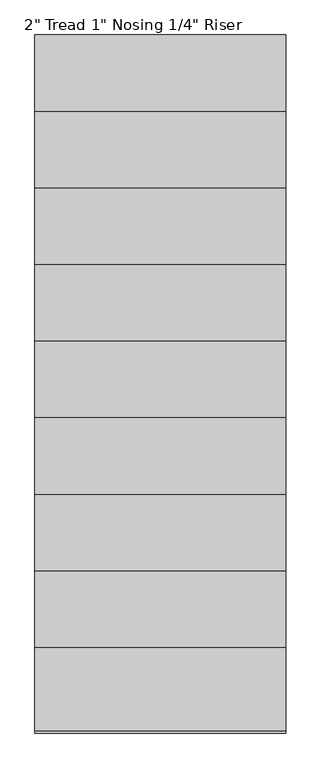
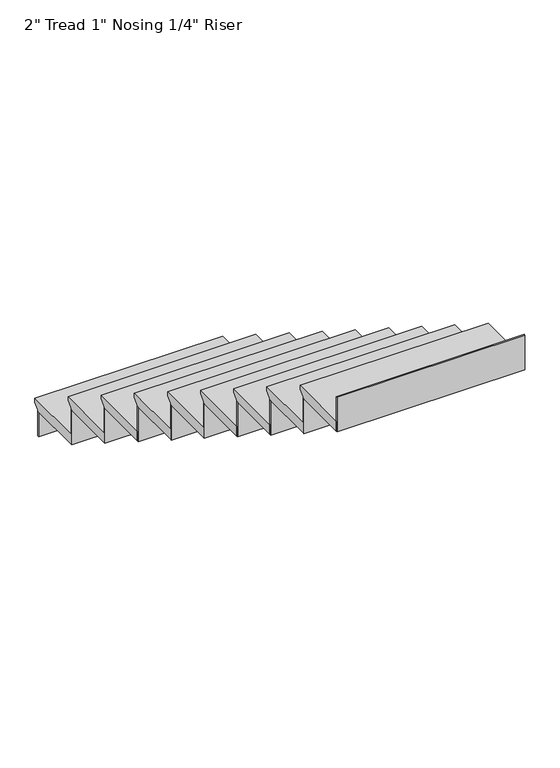
"""IFC4 building model written with IfcOpenShell, lengths in millimetres: stair flight geometry."""

from ifc_helpers import new_model, si_unit, origin, place, context, project, spatial, faceted_brep, source, transform, mapped, element, save


def stair_flight_2edfd720(model_context):
    return source(origin(), model_context, "Body", "Brep", [
        faceted_brep([(14235.8761273, -1100.1064015, 768.35), (14235.8761273, -1100.1064015, 787.4), (15150.2761273, -1100.1064015, 787.4), (15150.2761273, -1100.1064015, 768.35), (14235.8761273, -1125.5064015, 742.95), (15150.2761273, -1125.5064015, 742.95), (14235.8761273, -1404.9064015, 787.4), (15150.2761273, -1404.9064015, 787.4), (15150.2761273, -1125.5064015, 736.6), (15150.2761273, -1404.9064015, 736.6), (14235.8761273, -1404.9064015, 736.6), (14235.8761273, -1125.5064015, 736.6)], [[[0, 1, 2, 3]], [[4, 0, 3, 5]], [[2, 1, 6, 7]], [[8, 9, 10, 11]], [[2, 7, 9, 8, 5, 3]], [[8, 11, 4, 5]], [[6, 1, 0, 4, 11, 10]], [[7, 6, 10, 9]]]),
        faceted_brep([(14235.8761273, -1125.5064015, 736.6), (14235.8761273, -1125.5064015, 609.6), (14235.8761273, -1131.8564015, 609.6), (14235.8761273, -1131.8564015, 736.6), (15150.2761273, -1125.5064015, 736.6), (15150.2761273, -1131.8564015, 736.6), (15150.2761273, -1131.8564015, 609.6), (15150.2761273, -1125.5064015, 609.6)], [[[0, 1, 2, 3]], [[4, 5, 6, 7]], [[1, 0, 4, 7]], [[2, 1, 7, 6]], [[3, 2, 6, 5]], [[0, 3, 5, 4]]]),
        faceted_brep([(14235.8761273, -1404.9064015, 914.4), (14235.8761273, -1404.9064015, 736.6), (14235.8761273, -1411.2564015, 736.6), (14235.8761273, -1411.2564015, 914.4), (15150.2761273, -1404.9064015, 914.4), (15150.2761273, -1411.2564015, 914.4), (15150.2761273, -1411.2564015, 736.6), (15150.2761273, -1404.9064015, 736.6)], [[[0, 1, 2, 3]], [[4, 5, 6, 7]], [[1, 0, 4, 7]], [[2, 1, 7, 6]], [[3, 2, 6, 5]], [[0, 3, 5, 4]]]),
        faceted_brep([(15150.2761273, -1379.5064015, 965.2), (14235.8761273, -1379.5064015, 965.2), (14235.8761273, -1684.3064015, 965.2), (15150.2761273, -1684.3064015, 965.2), (15150.2761273, -1404.9064015, 914.4), (15150.2761273, -1684.3064015, 914.4), (14235.8761273, -1684.3064015, 914.4), (14235.8761273, -1404.9064015, 914.4), (15150.2761273, -1404.9064015, 920.75), (15150.2761273, -1379.5064015, 946.15), (14235.8761273, -1404.9064015, 920.75), (14235.8761273, -1379.5064015, 946.15)], [[[0, 1, 2, 3]], [[4, 5, 6, 7]], [[0, 3, 5, 4, 8, 9]], [[4, 7, 10, 8]], [[2, 1, 11, 10, 7, 6]], [[3, 2, 6, 5]], [[11, 1, 0, 9]], [[10, 11, 9, 8]]]),
        faceted_brep([(14235.8761273, -1684.3064015, 1092.2), (14235.8761273, -1684.3064015, 914.4), (14235.8761273, -1690.6564015, 914.4), (14235.8761273, -1690.6564015, 1092.2), (15150.2761273, -1684.3064015, 1092.2), (15150.2761273, -1690.6564015, 1092.2), (15150.2761273, -1690.6564015, 914.4), (15150.2761273, -1684.3064015, 914.4)], [[[0, 1, 2, 3]], [[4, 5, 6, 7]], [[1, 0, 4, 7]], [[2, 1, 7, 6]], [[3, 2, 6, 5]], [[0, 3, 5, 4]]]),
        faceted_brep([(15150.2761273, -1658.9064015, 1143.0), (14235.8761273, -1658.9064015, 1143.0), (14235.8761273, -1963.7064015, 1143.0), (15150.2761273, -1963.7064015, 1143.0), (15150.2761273, -1684.3064015, 1092.2), (15150.2761273, -1963.7064015, 1092.2), (14235.8761273, -1963.7064015, 1092.2), (14235.8761273, -1684.3064015, 1092.2), (15150.2761273, -1684.3064015, 1098.55), (15150.2761273, -1658.9064015, 1123.95), (14235.8761273, -1684.3064015, 1098.55), (14235.8761273, -1658.9064015, 1123.95)], [[[0, 1, 2, 3]], [[4, 5, 6, 7]], [[0, 3, 5, 4, 8, 9]], [[4, 7, 10, 8]], [[2, 1, 11, 10, 7, 6]], [[3, 2, 6, 5]], [[11, 1, 0, 9]], [[10, 11, 9, 8]]]),
        faceted_brep([(14235.8761273, -1963.7064015, 1270.0), (14235.8761273, -1963.7064015, 1092.2), (14235.8761273, -1970.0564015, 1092.2), (14235.8761273, -1970.0564015, 1270.0), (15150.2761273, -1963.7064015, 1270.0), (15150.2761273, -1970.0564015, 1270.0), (15150.2761273, -1970.0564015, 1092.2), (15150.2761273, -1963.7064015, 1092.2)], [[[0, 1, 2, 3]], [[4, 5, 6, 7]], [[1, 0, 4, 7]], [[2, 1, 7, 6]], [[3, 2, 6, 5]], [[0, 3, 5, 4]]]),
        faceted_brep([(15150.2761273, -1938.3064015, 1320.8), (14235.8761273, -1938.3064015, 1320.8), (14235.8761273, -2243.1064015, 1320.8), (15150.2761273, -2243.1064015, 1320.8), (15150.2761273, -1963.7064015, 1270.0), (15150.2761273, -2243.1064015, 1270.0), (14235.8761273, -2243.1064015, 1270.0), (14235.8761273, -1963.7064015, 1270.0), (15150.2761273, -1963.7064015, 1276.35), (15150.2761273, -1938.3064015, 1301.75), (14235.8761273, -1963.7064015, 1276.35), (14235.8761273, -1938.3064015, 1301.75)], [[[0, 1, 2, 3]], [[4, 5, 6, 7]], [[0, 3, 5, 4, 8, 9]], [[4, 7, 10, 8]], [[2, 1, 11, 10, 7, 6]], [[3, 2, 6, 5]], [[11, 1, 0, 9]], [[10, 11, 9, 8]]]),
        faceted_brep([(14235.8761273, -2243.1064015, 1447.8), (14235.8761273, -2243.1064015, 1270.0), (14235.8761273, -2249.4564015, 1270.0), (14235.8761273, -2249.4564015, 1447.8), (15150.2761273, -2243.1064015, 1447.8), (15150.2761273, -2249.4564015, 1447.8), (15150.2761273, -2249.4564015, 1270.0), (15150.2761273, -2243.1064015, 1270.0)], [[[0, 1, 2, 3]], [[4, 5, 6, 7]], [[1, 0, 4, 7]], [[2, 1, 7, 6]], [[3, 2, 6, 5]], [[0, 3, 5, 4]]]),
        faceted_brep([(15150.2761273, -2217.7064015, 1498.6), (14235.8761273, -2217.7064015, 1498.6), (14235.8761273, -2522.5064015, 1498.6), (15150.2761273, -2522.5064015, 1498.6), (15150.2761273, -2243.1064015, 1447.8), (15150.2761273, -2522.5064015, 1447.8), (14235.8761273, -2522.5064015, 1447.8), (14235.8761273, -2243.1064015, 1447.8), (15150.2761273, -2243.1064015, 1454.15), (15150.2761273, -2217.7064015, 1479.55), (14235.8761273, -2243.1064015, 1454.15), (14235.8761273, -2217.7064015, 1479.55)], [[[0, 1, 2, 3]], [[4, 5, 6, 7]], [[0, 3, 5, 4, 8, 9]], [[4, 7, 10, 8]], [[2, 1, 11, 10, 7, 6]], [[3, 2, 6, 5]], [[11, 1, 0, 9]], [[10, 11, 9, 8]]]),
        faceted_brep([(14235.8761273, -2522.5064015, 1625.6), (14235.8761273, -2522.5064015, 1447.8), (14235.8761273, -2528.8564015, 1447.8), (14235.8761273, -2528.8564015, 1625.6), (15150.2761273, -2522.5064015, 1625.6), (15150.2761273, -2528.8564015, 1625.6), (15150.2761273, -2528.8564015, 1447.8), (15150.2761273, -2522.5064015, 1447.8)], [[[0, 1, 2, 3]], [[4, 5, 6, 7]], [[1, 0, 4, 7]], [[2, 1, 7, 6]], [[3, 2, 6, 5]], [[0, 3, 5, 4]]]),
        faceted_brep([(15150.2761273, -2497.1064015, 1676.4), (14235.8761273, -2497.1064015, 1676.4), (14235.8761273, -2801.9064015, 1676.4), (15150.2761273, -2801.9064015, 1676.4), (15150.2761273, -2522.5064015, 1625.6), (15150.2761273, -2801.9064015, 1625.6), (14235.8761273, -2801.9064015, 1625.6), (14235.8761273, -2522.5064015, 1625.6), (15150.2761273, -2522.5064015, 1631.95), (15150.2761273, -2497.1064015, 1657.35), (14235.8761273, -2522.5064015, 1631.95), (14235.8761273, -2497.1064015, 1657.35)], [[[0, 1, 2, 3]], [[4, 5, 6, 7]], [[0, 3, 5, 4, 8, 9]], [[4, 7, 10, 8]], [[2, 1, 11, 10, 7, 6]], [[3, 2, 6, 5]], [[11, 1, 0, 9]], [[10, 11, 9, 8]]]),
        faceted_brep([(14235.8761273, -2801.9064015, 1803.4), (14235.8761273, -2801.9064015, 1625.6), (14235.8761273, -2808.2564015, 1625.6), (14235.8761273, -2808.2564015, 1803.4), (15150.2761273, -2801.9064015, 1803.4), (15150.2761273, -2808.2564015, 1803.4), (15150.2761273, -2808.2564015, 1625.6), (15150.2761273, -2801.9064015, 1625.6)], [[[0, 1, 2, 3]], [[4, 5, 6, 7]], [[1, 0, 4, 7]], [[2, 1, 7, 6]], [[3, 2, 6, 5]], [[0, 3, 5, 4]]]),
        faceted_brep([(15150.2761273, -2776.5064015, 1854.2), (14235.8761273, -2776.5064015, 1854.2), (14235.8761273, -3081.3064015, 1854.2), (15150.2761273, -3081.3064015, 1854.2), (15150.2761273, -2801.9064015, 1803.4), (15150.2761273, -3081.3064015, 1803.4), (14235.8761273, -3081.3064015, 1803.4), (14235.8761273, -2801.9064015, 1803.4), (15150.2761273, -2801.9064015, 1809.75), (15150.2761273, -2776.5064015, 1835.15), (14235.8761273, -2801.9064015, 1809.75), (14235.8761273, -2776.5064015, 1835.15)], [[[0, 1, 2, 3]], [[4, 5, 6, 7]], [[0, 3, 5, 4, 8, 9]], [[4, 7, 10, 8]], [[2, 1, 11, 10, 7, 6]], [[3, 2, 6, 5]], [[11, 1, 0, 9]], [[10, 11, 9, 8]]]),
        faceted_brep([(14235.8761273, -3081.3064015, 1981.2), (14235.8761273, -3081.3064015, 1803.4), (14235.8761273, -3087.6564015, 1803.4), (14235.8761273, -3087.6564015, 1981.2), (15150.2761273, -3081.3064015, 1981.2), (15150.2761273, -3087.6564015, 1981.2), (15150.2761273, -3087.6564015, 1803.4), (15150.2761273, -3081.3064015, 1803.4)], [[[0, 1, 2, 3]], [[4, 5, 6, 7]], [[1, 0, 4, 7]], [[2, 1, 7, 6]], [[3, 2, 6, 5]], [[0, 3, 5, 4]]]),
        faceted_brep([(15150.2761273, -3055.9064015, 2032.0), (14235.8761273, -3055.9064015, 2032.0), (14235.8761273, -3360.7064015, 2032.0), (15150.2761273, -3360.7064015, 2032.0), (15150.2761273, -3081.3064015, 1981.2), (15150.2761273, -3360.7064015, 1981.2), (14235.8761273, -3360.7064015, 1981.2), (14235.8761273, -3081.3064015, 1981.2), (15150.2761273, -3081.3064015, 1987.55), (15150.2761273, -3055.9064015, 2012.95), (14235.8761273, -3081.3064015, 1987.55), (14235.8761273, -3055.9064015, 2012.95)], [[[0, 1, 2, 3]], [[4, 5, 6, 7]], [[0, 3, 5, 4, 8, 9]], [[4, 7, 10, 8]], [[2, 1, 11, 10, 7, 6]], [[3, 2, 6, 5]], [[11, 1, 0, 9]], [[10, 11, 9, 8]]]),
        faceted_brep([(14235.8761273, -3640.1064015, 2336.8), (14235.8761273, -3640.1064015, 2159.0), (14235.8761273, -3646.4564015, 2159.0), (14235.8761273, -3646.4564015, 2336.8), (15150.2761273, -3640.1064015, 2336.8), (15150.2761273, -3646.4564015, 2336.8), (15150.2761273, -3646.4564015, 2159.0), (15150.2761273, -3640.1064015, 2159.0)], [[[0, 1, 2, 3]], [[4, 5, 6, 7]], [[1, 0, 4, 7]], [[2, 1, 7, 6]], [[3, 2, 6, 5]], [[0, 3, 5, 4]]]),
        faceted_brep([(14235.8761273, -3360.7064015, 2159.0), (14235.8761273, -3360.7064015, 1981.2), (14235.8761273, -3367.0564015, 1981.2), (14235.8761273, -3367.0564015, 2159.0), (15150.2761273, -3360.7064015, 2159.0), (15150.2761273, -3367.0564015, 2159.0), (15150.2761273, -3367.0564015, 1981.2), (15150.2761273, -3360.7064015, 1981.2)], [[[0, 1, 2, 3]], [[4, 5, 6, 7]], [[1, 0, 4, 7]], [[2, 1, 7, 6]], [[3, 2, 6, 5]], [[0, 3, 5, 4]]]),
        faceted_brep([(15150.2761273, -3640.1064015, 2209.8), (15150.2761273, -3614.7064015, 2209.8), (15150.2761273, -3335.3064015, 2209.8), (14235.8761273, -3335.3064015, 2209.8), (14235.8761273, -3640.1064015, 2209.8), (15150.2761273, -3614.7064015, 2159.0), (15150.2761273, -3640.1064015, 2159.0), (14235.8761273, -3640.1064015, 2159.0), (14235.8761273, -3360.7064015, 2159.0), (15150.2761273, -3360.7064015, 2159.0), (15150.2761273, -3360.7064015, 2165.35), (15150.2761273, -3335.3064015, 2190.75), (14235.8761273, -3360.7064015, 2165.35), (14235.8761273, -3335.3064015, 2190.75)], [[[0, 1, 2, 3, 4]], [[5, 6, 7, 8, 9]], [[1, 0, 6, 5]], [[2, 1, 5, 9, 10, 11]], [[9, 8, 12, 10]], [[4, 3, 13, 12, 8, 7]], [[0, 4, 7, 6]], [[13, 3, 2, 11]], [[12, 13, 11, 10]]]),
    ])


if __name__ == "__main__":
    model = new_model("IFC4")
    model_context = context("Model", 3, world=origin())
    ifc_project = project(units=[si_unit("LENGTHUNIT", "METRE", prefix="MILLI")], contexts=[model_context])
    site = spatial("IfcSite", under=ifc_project)
    building = spatial("IfcBuilding", under=site)
    placement = place(None, origin())
    stair_flight_shape = stair_flight_2edfd720(model_context)
    element("IfcStairFlight", 1, ObjectType="2\" Tread 1\" Nosing 1/4\" Riser", at=placement, inside=building, context=model_context, shape_type="MappedRepresentation", body=[
        mapped(stair_flight_shape, transform((0.0, 0.0, 0.0), x_axis=(1.0, 0.0, 0.0), y_axis=(0.0, 1.0, 0.0), z_axis=(0.0, 0.0, 1.0))),
    ])
    save(model, "model.ifc")
